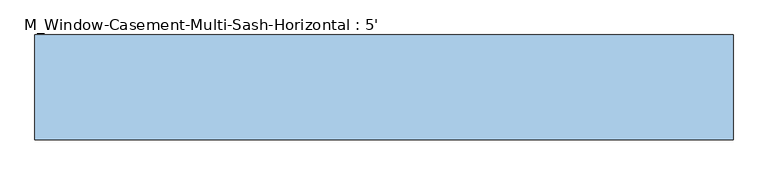
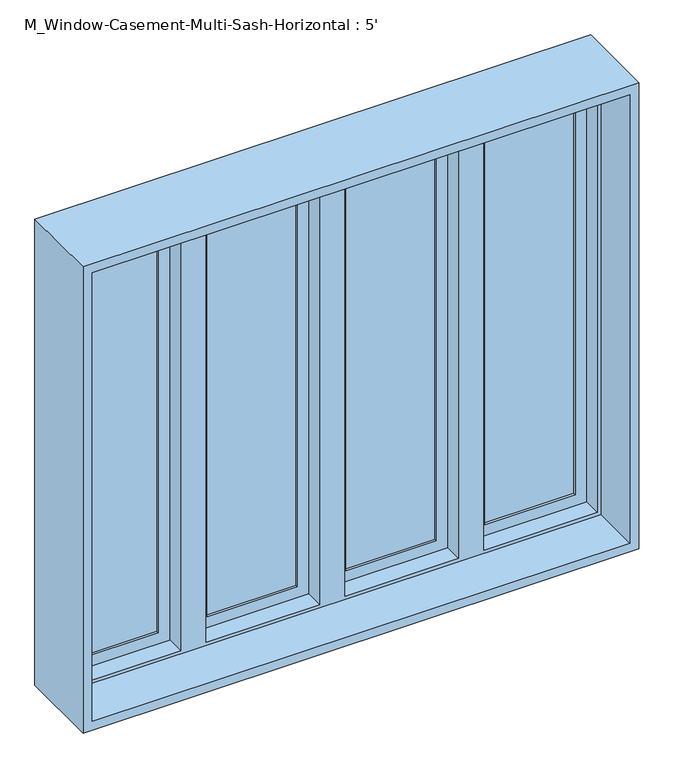
"""IFC4 building model written with IfcOpenShell, lengths in millimetres: window geometry, M_Window-Casement-Multi-Sash-Horizontal : 5'."""

from ifc_helpers import new_model, si_unit, frame, origin, place, context, project, spatial, polyline, outline, extrude, faceted_brep, source, transform, mapped, element, save


def m_window_casement_multi_sash_horizontal_5_4f9d37b3(model_context):
    return source(origin(), model_context, "Body", "SolidModel", [
        extrude(outline(polyline([(2224.6, 406.4), (925.4, 406.4), (925.4, 736.6), (2224.6, 736.6), (2224.6, 406.4)]), holes=[polyline([(2183.2, 695.2), (966.8, 695.2), (966.8, 447.8), (2183.2, 447.8), (2183.2, 695.2)])]), frame((0.0, 73.0, 0.0), z_axis=(0.0, 1.0, 0.0), x_axis=(0.0, 0.0, 1.0)), (0.0, 0.0, 1.0), 31.75),
        extrude(outline(polyline([(2224.6, -736.6), (925.4, -736.6), (925.4, -406.4), (2224.6, -406.4), (2224.6, -736.6)]), holes=[polyline([(2183.2, -447.8), (966.8, -447.8), (966.8, -695.2), (2183.2, -695.2), (2183.2, -447.8)])]), frame((0.0, 73.0, 0.0), z_axis=(0.0, 1.0, 0.0), x_axis=(0.0, 0.0, 1.0)), (0.0, 0.0, 1.0), 31.75),
        extrude(outline(polyline([(-447.8, 98.4), (-447.8, 92.05), (-695.2, 92.05), (-695.2, 98.4), (-447.8, 98.4)])), frame((0.0, 0.0, 967.2703125), z_axis=(0.0, 0.0, 1.0), x_axis=(1.0, 0.0, 0.0)), (0.0, 0.0, 1.0), 1215.9296875),
        extrude(outline(polyline([(-447.8, 85.7), (-447.8, 79.35), (-695.2, 79.35), (-695.2, 85.7), (-447.8, 85.7)])), frame((0.0, 0.0, 967.2703125), z_axis=(0.0, 0.0, 1.0), x_axis=(1.0, 0.0, 0.0)), (0.0, 0.0, 1.0), 1215.9296875),
        extrude(outline(polyline([(695.2, 98.4), (695.2, 92.05), (447.8, 92.05), (447.8, 98.4), (695.2, 98.4)])), frame((0.0, 0.0, 967.2703125), z_axis=(0.0, 0.0, 1.0), x_axis=(1.0, 0.0, 0.0)), (0.0, 0.0, 1.0), 1215.9296875),
        extrude(outline(polyline([(695.2, 85.7), (695.2, 79.35), (447.8, 79.35), (447.8, 85.7), (695.2, 85.7)])), frame((0.0, 0.0, 967.2703125), z_axis=(0.0, 0.0, 1.0), x_axis=(1.0, 0.0, 0.0)), (0.0, 0.0, 1.0), 1215.9296875),
        extrude(outline(polyline([(-66.8, 98.4), (-66.8, 92.05), (-314.2, 92.05), (-314.2, 98.4), (-66.8, 98.4)])), frame((0.0, 0.0, 966.8), z_axis=(0.0, 0.0, 1.0), x_axis=(1.0, 0.0, 0.0)), (0.0, 0.0, 1.0), 1216.4),
        extrude(outline(polyline([(-66.8, 85.7), (-66.8, 79.35), (-314.2, 79.35), (-314.2, 85.7), (-66.8, 85.7)])), frame((0.0, 0.0, 966.8), z_axis=(0.0, 0.0, 1.0), x_axis=(1.0, 0.0, 0.0)), (0.0, 0.0, 1.0), 1216.4),
        extrude(outline(polyline([(314.2, 98.4), (314.2, 92.05), (66.8, 92.05), (66.8, 98.4), (314.2, 98.4)])), frame((0.0, 0.0, 966.8), z_axis=(0.0, 0.0, 1.0), x_axis=(1.0, 0.0, 0.0)), (0.0, 0.0, 1.0), 1216.4),
        extrude(outline(polyline([(314.2, 85.7), (314.2, 79.35), (66.8, 79.35), (66.8, 85.7), (314.2, 85.7)])), frame((0.0, 0.0, 966.8), z_axis=(0.0, 0.0, 1.0), x_axis=(1.0, 0.0, 0.0)), (0.0, 0.0, 1.0), 1216.4),
        faceted_brep([(-406.4, 73.0, 2224.6), (-736.6, 73.0, 2224.6), (-736.6, 114.3, 2224.6), (736.6, 114.3, 2224.6), (736.6, 73.0, 2224.6), (406.4, 73.0, 2224.6), (406.4, 111.1, 2224.6), (355.6, 111.1, 2224.6), (355.6, 73.0, 2224.6), (25.4, 73.0, 2224.6), (25.4, 111.1, 2224.6), (-25.4, 111.1, 2224.6), (-25.4, 73.0, 2224.6), (-355.6, 73.0, 2224.6), (-355.6, 111.1, 2224.6), (-406.4, 111.1, 2224.6), (-727.0, 22.2, 2215.0), (-727.0, 73.0, 2215.0), (-416.0, 73.0, 2215.0), (-416.0, 22.2, 2215.0), (727.0, 73.0, 2215.0), (727.0, 22.2, 2215.0), (416.0, 22.2, 2215.0), (416.0, 73.0, 2215.0), (-346.0, 73.0, 2215.0), (-35.0, 73.0, 2215.0), (-35.0, 22.2, 2215.0), (-346.0, 22.2, 2215.0), (35.0, 73.0, 2215.0), (346.0, 73.0, 2215.0), (346.0, 22.2, 2215.0), (35.0, 22.2, 2215.0), (-736.6, -114.3, 2224.6), (-736.6, 22.2, 2224.6), (736.6, 22.2, 2224.6), (736.6, -114.3, 2224.6), (-762.0, 114.3, 2250.0), (-762.0, -114.3, 2250.0), (762.0, -114.3, 2250.0), (762.0, 114.3, 2250.0), (736.6, 114.3, 925.4), (736.6, 73.0, 925.4), (727.0, 73.0, 935.0), (727.0, 22.2, 935.0), (736.6, 22.2, 925.4), (736.6, -114.3, 925.4), (762.0, -114.3, 900.0), (762.0, 114.3, 900.0), (406.4, 73.0, 925.4), (-736.6, 114.3, 925.4), (-736.6, 73.0, 925.4), (-406.4, 73.0, 925.4), (-406.4, 111.1, 925.4), (-355.6, 111.1, 925.4), (-355.6, 73.0, 925.4), (-25.4, 73.0, 925.4), (-25.4, 111.1, 925.4), (25.4, 111.1, 925.4), (25.4, 73.0, 925.4), (355.6, 73.0, 925.4), (355.6, 111.1, 925.4), (406.4, 111.1, 925.4), (416.0, 73.0, 935.0), (416.0, 22.2, 935.0), (-727.0, 73.0, 935.0), (-727.0, 22.2, 935.0), (-416.0, 22.2, 935.0), (-416.0, 73.0, 935.0), (-35.0, 73.0, 935.0), (-346.0, 73.0, 935.0), (-346.0, 22.2, 935.0), (-35.0, 22.2, 935.0), (346.0, 73.0, 935.0), (35.0, 73.0, 935.0), (35.0, 22.2, 935.0), (346.0, 22.2, 935.0), (-736.6, 22.2, 925.4), (-736.6, -114.3, 925.4), (-762.0, -114.3, 900.0), (-762.0, 114.3, 900.0)], [[[0, 1, 2, 3, 4, 5, 6, 7, 8, 9, 10, 11, 12, 13, 14, 15]], [[16, 17, 18, 19]], [[20, 21, 22, 23]], [[24, 25, 26, 27]], [[28, 29, 30, 31]], [[32, 33, 34, 35]], [[36, 37, 38, 39]], [[4, 3, 40, 41]], [[21, 20, 42, 43]], [[35, 34, 44, 45]], [[39, 38, 46, 47]], [[48, 41, 40, 49, 50, 51, 52, 53, 54, 55, 56, 57, 58, 59, 60, 61]], [[43, 42, 62, 63]], [[64, 65, 66, 67]], [[68, 69, 70, 71]], [[72, 73, 74, 75]], [[45, 44, 76, 77]], [[47, 46, 78, 79]], [[2, 1, 50, 49]], [[4, 41, 48, 5], [20, 23, 62, 42]], [[50, 1, 0, 51], [64, 67, 18, 17]], [[12, 55, 54, 13], [69, 68, 25, 24]], [[8, 59, 58, 9], [73, 72, 29, 28]], [[17, 16, 65, 64]], [[44, 34, 33, 76], [16, 19, 66, 65], [27, 26, 71, 70], [31, 30, 75, 74], [21, 43, 63, 22]], [[33, 32, 77, 76]], [[38, 37, 78, 46], [32, 35, 45, 77]], [[37, 36, 79, 78]], [[36, 39, 47, 79], [3, 2, 49, 40]], [[18, 67, 66, 19]], [[69, 24, 27, 70]], [[53, 14, 13, 54]], [[14, 53, 52, 15]], [[15, 52, 51, 0]], [[25, 68, 71, 26]], [[73, 28, 31, 74]], [[57, 10, 9, 58]], [[10, 57, 56, 11]], [[11, 56, 55, 12]], [[6, 61, 60, 7]], [[7, 60, 59, 8]], [[29, 72, 75, 30]], [[62, 23, 22, 63]], [[61, 6, 5, 48]]]),
        extrude(outline(polyline([(2224.6, 25.4), (925.4, 25.4), (925.4, 355.6), (2224.6, 355.6), (2224.6, 25.4)]), holes=[polyline([(2183.2, 314.2), (966.8, 314.2), (966.8, 66.8), (2183.2, 66.8), (2183.2, 314.2)])]), frame((0.0, 73.0, 0.0), z_axis=(0.0, 1.0, 0.0), x_axis=(0.0, 0.0, 1.0)), (0.0, 0.0, 1.0), 31.75),
        extrude(outline(polyline([(2224.6, -355.6), (925.4, -355.6), (925.4, -25.4), (2224.6, -25.4), (2224.6, -355.6)]), holes=[polyline([(2183.2, -66.8), (966.8, -66.8), (966.8, -314.2), (2183.2, -314.2), (2183.2, -66.8)])]), frame((0.0, 73.0, 0.0), z_axis=(0.0, 1.0, 0.0), x_axis=(0.0, 0.0, 1.0)), (0.0, 0.0, 1.0), 31.75),
    ])


if __name__ == "__main__":
    model = new_model("IFC4")
    model_context = context("Model", 3, world=origin())
    ifc_project = project(units=[si_unit("LENGTHUNIT", "METRE", prefix="MILLI")], contexts=[model_context])
    site = spatial("IfcSite", under=ifc_project)
    building = spatial("IfcBuilding", under=site)
    placement = place(None, origin())
    m_window_casement_multi_sash_horizontal_5_shape = m_window_casement_multi_sash_horizontal_5_4f9d37b3(model_context)
    element("IfcWindow", 1, ObjectType="M_Window-Casement-Multi-Sash-Horizontal : 5'", at=placement, inside=building, context=model_context, shape_type="MappedRepresentation", body=[
        mapped(m_window_casement_multi_sash_horizontal_5_shape, transform((0.0, 0.0, 0.0), x_axis=(1.0, 0.0, 0.0), y_axis=(0.0, 1.0, 0.0), z_axis=(0.0, 0.0, 1.0))),
    ])
    save(model, "model.ifc")

# Revit data of these elements
# Type "M_Window-Casement-Multi-Sash-Horizontal : 5'"
#   Type Mark = "32"
#   Fire Rating = "0.5h"
#   Assembly Code = "B2020100"
#   Analytic Construction = "Double glazing - domestic"
#   Window Inset [instance default] = 0' - 0.62598"
#   Wall Thickness [instance default] = 0' - 5.90551"
#   Visual Light Transmittance = 0.81
#   Thermal Resistance (R) = 0.319569 (m²·K)/W
#   Solar Heat Gain Coefficient = 0.76
#   Rough Width = 5' - 0.59055"
#   Rough Height = 4' - 5.74016"
#   Open Window Width = 1' - 3"
#   Heat Transfer Coefficient (U) = 3.12929 W/(m²·K)
#   Height = 4' - 5.14961"
#   Frame Gap 3 [instance default] = 0' - 1.62992"
#   Frame Gap 2 [instance default] = 0' - 0.62598"
#   Frame Gap 1 = 0' - 1.37795"
#   Default Sill Height = 2' - 11.43307"
#   Width = 5' - 0"
#   Frame Material = Metal - Aluminum
#   Glass Panel Material = Glass
#   Wall Closure = (empty or 0)
# Element 1 (IfcWindow, "M_Window-Casement-Multi-Sash-Horizontal : 5'")
#   Wall Thickness = 0' - 9"
#   Materials on its faces: "Metal - Aluminum", "Glass"
# Materials
#   "Metal - Aluminum": class "Metal", colour RGB 247 247 247, transparency 0
#   "Glass": class "Glass", colour RGB 0 128 192, transparency 0.9, Description = "Soda Lime Glass", Cost = 0
